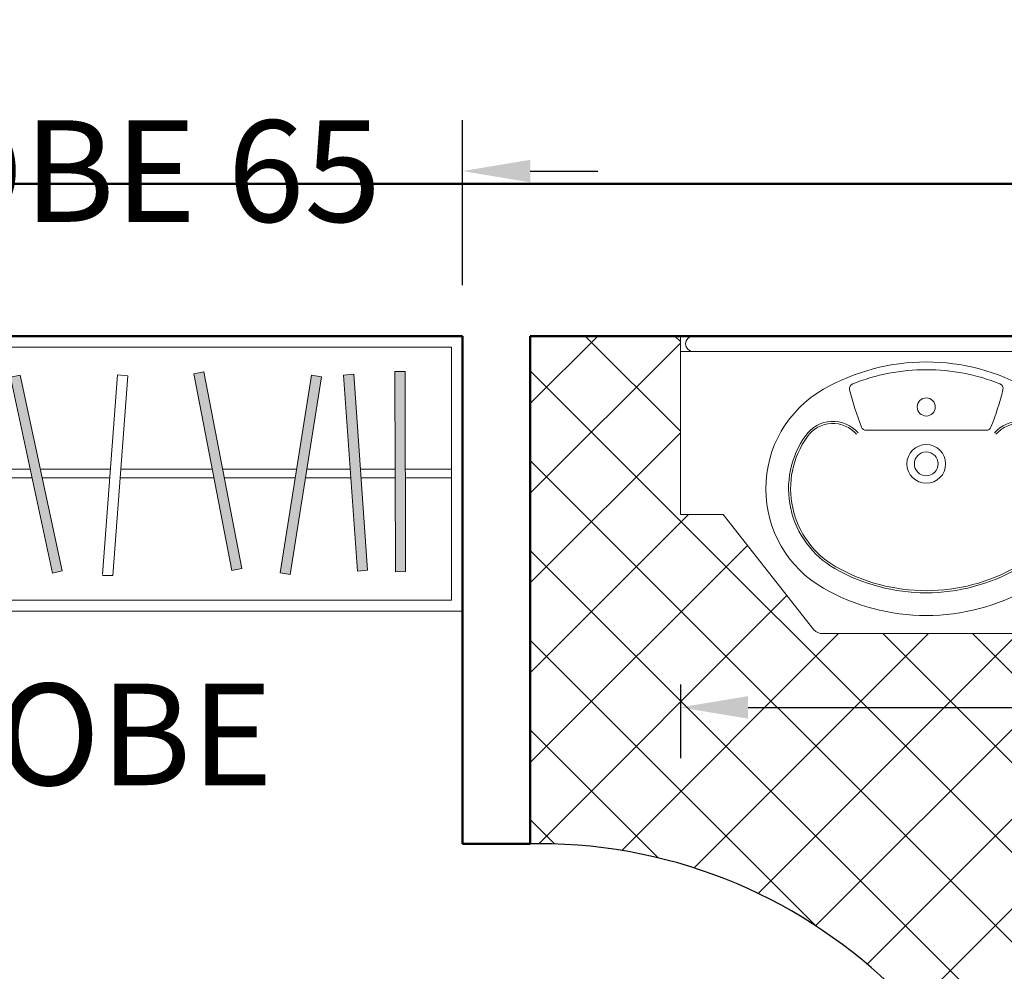
# Model space of a CAD drawing. Units: inches. Extents: x -466983 to 1020, y 324 to 318697.
# Tile 47 of 97: x 491 to 549, y 1038 to 1095. Entities that reach past the tile are written whole.
import ezdxf

# ---------------------------------------------------------------- set-up
doc = ezdxf.new("R2010")
doc.units = ezdxf.units.IN
doc.header["$MEASUREMENT"] = 0
for name, color, linetype, lineweight in [('A-ANNO-DIMS', 2, 'Continuous', 18), ('A-ANNO-TEXT', 7, 'Continuous', 18), ('A-DOOR', 3, 'Continuous', 25), ('A-FLOR-FIXT', 9, 'Continuous', 18), ('A-FLOR-PATT', 252, 'Continuous', 13), ('A-FURN', 8, 'Continuous', 18), ('A-WALL', 7, 'Continuous', 50)]:
    doc.layers.add(name, color=color, linetype=linetype, lineweight=lineweight)
doc.styles.get("Standard").update_dxf_attribs({"font": 'arial.ttf'})
doc.dimstyles.get("Standard").update_dxf_attribs({"dimtxt": 6, "dimasz": 4, "dimexe": 3, "dimexo": 3, "dimgap": 0.09, "dimtad": 0, "dimtih": 1, "dimtoh": 1, "dimdec": 1, "dimzin": 0, "dimdsep": 46, "dimlunit": 3, "dimtxsty": 'Standard', "dimcen": 0.09, "dimadec": 0, "dimazin": 0, "dimtfac": 1, "dimtdec": 1, "dimtofl": 0, "dimtmove": 0, "dimatfit": 3, "dimfxl": 1, "dimtolj": 1, "dimtzin": 0, "dimarcsym": 0})

# ---------------------------------------------------------------- blocks, each defined once
blk = doc.blocks.new('*U38')
for p, q in [((0, 0), (-1.1e-15, 5.999999999999999)), ((40, 8e-15), (40, 6.000000000000007))]:
    blk.add_line(p, q)
blk.add_lwpolyline([(0, 0), (1.42e-14, -40), (1.750000000000014, -40), (1.75, 9e-16)], close=True)
blk.add_arc((0, 0), 40, 270, 0)
blk = doc.blocks.new('B3')
for p, q in [((-450, 0), (-455.7402514854766, -1.1418070123309)), ((450, 0), (455.7402514854766, -1.1418070123309)), ((-463.8581929876745, -9.25974851452338), (-465, -15)), ((-465, -15), (-463.8581929876745, -20.74025148547662)), ((-460.6066017178018, -4.393398282201815), (-463.8581929876745, -9.25974851452338)), ((-455.7402514854766, -1.1418070123309), (-460.6066017178018, -4.393398282201815)), ((455.7402514854766, -1.1418070123309), (460.6066017177945, -4.393398282201815)), ((460.6066017177945, -4.393398282201815), (463.8581929876672, -9.25974851452338)), ((463.8581929876672, -9.25974851452338), (465, -15)), ((465, -15), (463.8581929876672, -20.74025148547662)), ((475, -30), (-475, -30)), ((-463.8581929876745, -20.74025148547662), (-460.6066017178018, -25.60660171779819)), ((-460.6066017178018, -25.60660171779819), (-455.7402514854766, -28.8581929876691)), ((-455.7402514854766, -28.8581929876691), (-450, -30)), ((455.7402514854766, -28.8581929876691), (450, -30)), ((460.6066017177945, -25.60660171779819), (455.7402514854766, -28.8581929876691)), ((463.8581929876672, -20.74025148547662), (460.6066017177945, -25.60660171779819)), ((2.91038e-11, -182.0000000000054), (-115.8117069986983, -182.0000000000054)), ((2.91038e-11, -182.0000000000054), (115.8117069987565, -182.0000000000054))]:
    blk.add_line(p, q)
blk.add_lwpolyline([(199.4833683843535, -575, 0.2017697719241106), (217.3542190239823, -567.482353886593), (392.5, -345), (435, -345), (475, -345), (475, 0), (-475, 0), (-475, -345), (-435, -345), (-392.5, -345), (-217.3542190239896, -567.482353886593, 0.2017697719241107), (-199.4833683843608, -575)], format="xyb", close=True)
for centre, radius, start, end in [((5.09317e-11, -450.0000000000327), 400.0000000000322, 90, 119.7172288959075), ((0, -450.0000000000327), 400.0000000000319, 60.28277110409252, 90), ((2.91038e-11, -450.0000000000055), 385, 90, 111.6513567404431), ((2.91038e-11, -450.0000000000055), 385, 68.34864325955687, 90), ((-138.3591766736499, -101.4576952073475), 10, 111.6513567404431, 193.3915177581575), ((138.3591766737008, -101.4576952073475), 10, 346.6084822418425, 68.34864325955687), ((-88.47222222221171, -295.0000000000055), 221.527777777762, 119.7172288959075, 240.2827711040925), ((338.3178096717893, 12.0282100348104), 500, 193.3915177581575, 202.0594091764406), ((-338.3178096717383, 12.0282100348104), 500, 337.9405908235594, 346.6084822418425), ((88.47222222225537, -294.9999999999964), 221.527777777762, 299.7172288959074, 60.28277110409252), ((2.91038e-11, -136.9999999999891), 17.5, 90, 270), ((2.91038e-11, -136.9999999999891), 17.5, 270, 90), ((-180.5137974189128, -229.2550553338115), 64.41699441097052, 40.71477974361456, 144.4619255202982), ((-180.5137974189128, -229.2550553338115), 60.41699441097051, 40.71477974361456, 144.4619255202982), ((180.5137974189638, -229.2550553338115), 64.41699441097052, 35.53807447970174, 139.2852202563854), ((180.5137974189638, -229.2550553338115), 60.41699441097051, 35.53807447970174, 139.2852202563854), ((-115.8117069986983, -172.0000000000145), 10, 202.0594091764406, 270), ((115.8117069987565, -172.0000000000145), 10, 270, 337.9405908235594), ((-88.47222222221171, -295.0000000000055), 177.5277777777778, 144.4619255202982, 240.2827711040925), ((-88.47222222221171, -295.0000000000055), 173.5277777777778, 144.4619255202982, 240.2827711040925), ((88.47222222223354, -295.0000000000055), 173.5277777777778, 299.7172288959074, 35.53807447970174), ((88.47222222223354, -295.0000000000055), 177.5277777777778, 299.7172288959074, 35.53807447970174), ((2.91038e-11, -247.0000000000037), 37.5, 90, 270), ((2.91038e-11, -247.0000000000037), 23, 90, 270), ((2.91038e-11, -247.0000000000037), 37.5, 270, 90), ((2.91038e-11, -247.0000000000037), 23, 270, 90), ((2.91038e-11, -140.0000000000036), 356, 240.2827711040925, 270), ((2.91038e-11, -140.0000000000036), 352, 240.2827711040925, 270), ((2.91038e-11, -140.0000000000036), 352, 270, 299.7172288959074), ((2.91038e-11, -140.0000000000036), 356, 270, 299.7172288959074), ((5.09317e-11, -139.9999999999781), 400.0000000000309, 240.2827711040925, 270), ((-1.45519e-11, -140.0000000000309), 399.9999999999781, 270, 299.7172288959074)]:
    blk.add_arc(centre, radius, start, end)
blk = doc.blocks.new('Wardrobe 1.1')
h = blk.add_hatch(color=256)
h.dxf.hatch_style = 1
h.paths.add_polyline_path([(4623.63130591675, 1559.127828082639), (4605.452274823494, 1555.618178042687), (4674.43862754123, 1198.026895294012), (4692.617658634486, 1201.536545333964)])
h = blk.add_hatch(color=256)
h.dxf.hatch_style = 1
h.paths.add_polyline_path([(4989.37316691601, 1559.911022331437), (4970.858516418657, 1559.860704815934), (4971.798831744867, 1195.677017418713), (4990.313482242336, 1195.727334934216)])
h = blk.add_hatch(color=256)
h.dxf.hatch_style = 1
h.paths.add_polyline_path([(3151.282105115228, 1187.510288244974), (3169.796885531561, 1187.510288244974), (3168.856570205235, 1551.693975642194), (3150.341919707882, 1551.643658126692)])
h = blk.add_hatch(color=256)
h.dxf.hatch_style = 1
h.paths.add_polyline_path([(3361.868584936534, 1541.669378461711), (3343.939726713163, 1546.290077294676), (3253.002619132332, 1193.641406768397), (3270.931477355587, 1189.02070793549)])
h = blk.add_hatch(color=256)
h.dxf.hatch_style = 1
h.paths.add_polyline_path([(3403.891248248334, 1551.693975642194), (3385.376597750981, 1551.643658126692), (3386.316913077191, 1187.459970729471), (3404.831563574544, 1187.510288244974)])
h = blk.add_hatch(color=256)
h.dxf.hatch_style = 1
h.paths.add_polyline_path([(3596.9032629794, 1541.669378461711), (3578.974404756262, 1546.290077294676), (3488.037297175316, 1193.641406768397), (3505.966155398454, 1189.02070793549)])
h = blk.add_hatch(color=256)
h.dxf.hatch_style = 1
h.paths.add_polyline_path([(3664.213577620618, 1553.074679382599), (3646.111361609239, 1549.18821693327), (3722.509827192224, 1193.106882382172), (3740.612043203603, 1196.993344831501)])
h = blk.add_hatch(color=256)
h.dxf.hatch_style = 1
h.paths.add_polyline_path([(3813.833679657712, 1190.320201264565), (3832.296488257873, 1188.934736184298), (3859.597907476409, 1552.094859088468), (3841.135098876248, 1553.480324168735)])
h = blk.add_hatch(color=256)
h.dxf.hatch_style = 1
h.paths.add_polyline_path([(4029.392729275909, 1551.693975642194), (4010.878078778556, 1551.643658126692), (4011.818394104767, 1187.459970729471), (4030.333044602236, 1187.510288244974)])
h = blk.add_hatch(color=256)
h.dxf.hatch_style = 1
h.paths.add_polyline_path([(4222.404744007092, 1541.669378461711), (4204.475885783836, 1546.290077294676), (4113.538778203007, 1193.641406768397), (4131.467636426145, 1189.02070793549)])
h = blk.add_hatch(color=256)
h.dxf.hatch_style = 1
h.paths.add_polyline_path([(4348.011308219915, 1193.106882382172), (4366.113524231294, 1196.993344831501), (4289.715058648309, 1553.074679382599), (4271.612842636931, 1549.18821693327)])
h = blk.add_hatch(color=256)
h.dxf.hatch_style = 1
h.paths.add_polyline_path([(4837.600952654661, 1550.260731044678), (4819.316543353771, 1553.17194924514), (4762.004005428219, 1193.525017719703), (4780.288414729109, 1190.613799519242)])
h = blk.add_hatch(color=256)
h.dxf.hatch_style = 1
h.paths.add_polyline_path([(4895.873954488479, 1554.659198605851), (4877.410424046501, 1553.283386659738), (4902.671188982951, 1196.772307061869), (4921.13471942493, 1198.148119007923)])
at = {"ltscale": 5}
for p, q in [((3093.82979383441, 1124.111993690416), (3093.82979383441, 1624.111993690416)), ((3093.82979383441, 1624.111993690416), (5093.829793834409, 1624.111993690416)), ((5093.829793834409, 1624.111993690416), (5093.829793834409, 1124.111993690416)), ((5093.829793834409, 1124.111993690416), (3093.82979383441, 1124.111993690416))]:
    blk.add_line(p, q, dxfattribs=at)
for p, q in [((3113.82979383441, 1144.111993690416), (3113.82979383441, 1604.111993690416)), ((3113.82979383441, 1604.111993690416), (5073.829793834409, 1604.111993690416)), ((5073.829793834409, 1604.111993690416), (5073.829793834409, 1144.111993690416)), ((4623.63130591675, 1559.127828082639), (4605.452274823494, 1555.618178042687)), ((4692.617658634486, 1201.536545333964), (4623.63130591675, 1559.127828082639)), ((4989.37316691601, 1559.911022331437), (4970.858516418657, 1559.860704815934)), ((4970.858516418657, 1559.860704815934), (4971.798831744867, 1195.677017418713)), ((4990.313482242336, 1195.727334934216), (4989.37316691601, 1559.911022331437)), ((3168.856570205235, 1551.693975642194), (3150.341919707882, 1551.643658126692)), ((3150.341919707882, 1551.643658126692), (3151.282235034092, 1187.459970729471)), ((3169.796885531561, 1187.510288244974), (3168.856570205235, 1551.693975642194)), ((3343.939726713163, 1546.290077294676), (3253.002619132332, 1193.641406768397)), ((3270.931477355587, 1189.02070793549), (3361.868584936534, 1541.669378461711)), ((3361.868584936534, 1541.669378461711), (3343.939726713163, 1546.290077294676)), ((3403.891248248334, 1551.693975642194), (3385.376597750981, 1551.643658126692)), ((3385.376597750981, 1551.643658126692), (3386.316913077191, 1187.459970729471)), ((3404.831563574544, 1187.510288244974), (3403.891248248334, 1551.693975642194)), ((3578.974404756262, 1546.290077294676), (3488.037297175316, 1193.641406768397)), ((3505.966155398454, 1189.02070793549), (3596.9032629794, 1541.669378461711)), ((3596.9032629794, 1541.669378461711), (3578.974404756262, 1546.290077294676)), ((3664.213577620618, 1553.074679382599), (3646.111361609239, 1549.18821693327)), ((3646.111361609239, 1549.18821693327), (3722.509827192224, 1193.106882382172)), ((3740.612043203603, 1196.993344831501), (3664.213577620618, 1553.074679382599)), ((3841.135098876248, 1553.480324168735), (3813.833679657712, 1190.320201264565)), ((3832.296488257873, 1188.934736184298), (3859.597907476409, 1552.094859088468)), ((3859.597907476409, 1552.094859088468), (3841.135098876248, 1553.480324168735)), ((4029.392729275909, 1551.693975642194), (4010.878078778556, 1551.643658126692)), ((4010.878078778556, 1551.643658126692), (4011.818394104767, 1187.459970729471)), ((4030.333044602236, 1187.510288244974), (4029.392729275909, 1551.693975642194)), ((4204.475885783836, 1546.290077294676), (4113.538778203007, 1193.641406768397)), ((4131.467636426145, 1189.02070793549), (4222.404744007092, 1541.669378461711)), ((4222.404744007092, 1541.669378461711), (4204.475885783836, 1546.290077294676)), ((4289.715058648309, 1553.074679382599), (4271.612842636931, 1549.18821693327)), ((4271.612842636931, 1549.18821693327), (4348.011308219915, 1193.106882382172)), ((4366.113524231294, 1196.993344831501), (4289.715058648309, 1553.074679382599)), ((4605.452274823494, 1555.618178042687), (4674.43862754123, 1198.026895294012)), ((4819.316543353771, 1553.17194924514), (4762.004005428219, 1193.525017719703)), ((4780.288414729109, 1190.613799519242), (4837.600952654661, 1550.260731044678)), ((4837.600952654661, 1550.260731044678), (4819.316543353771, 1553.17194924514)), ((4895.873954488479, 1554.659198605851), (4877.410424046501, 1553.283386659738)), ((4877.410424046501, 1553.283386659738), (4902.671188982951, 1196.772307061869)), ((4921.13471942493, 1198.148119007923), (4895.873954488479, 1554.659198605851)), ((3150.779647227988, 1382.111993690416), (3113.82979383441, 1382.111993690416)), ((3301.603312885615, 1382.111993690416), (3169.294427644258, 1382.111993690416)), ((3301.603312885671, 1382.111993690416), (3169.294427644278, 1382.111993690416)), ((3385.814325271087, 1382.111993690416), (3320.723705409183, 1382.111993690416)), ((3536.63799092866, 1382.111993690416), (3404.329105687303, 1382.111993690416)), ((3536.637990928537, 1382.111993690416), (3404.329105687377, 1382.111993690416)), ((3681.958135513426, 1382.111993690416), (3555.75838345205, 1382.111993690416)), ((3681.958135513406, 1382.111993690416), (3555.758383452127, 1382.111993690416)), ((3828.252080240405, 1382.111993690416), (3700.894205307252, 1382.111993690416)), ((3828.252080240453, 1382.111993690416), (3700.894205307288, 1382.111993690416)), ((4011.315806298681, 1382.111993690416), (3846.819044447374, 1382.111993690416)), ((4162.139471956229, 1382.111993690416), (4029.830586714952, 1382.111993690416)), ((4307.459616541096, 1382.111993690416), (4181.259864479818, 1382.111993690416)), ((4453.753561268143, 1382.111993690416), (4326.395686334979, 1382.111993690416)), ((4638.925011464094, 1382.111993690416), (4472.320525475011, 1382.111993690416)), ((4792.056807955193, 1382.111993690416), (4657.781122696752, 1382.111993690416)), ((4889.538855865531, 1382.111993690416), (4810.805142536459, 1382.111993690416)), ((4971.317460196375, 1382.111993690416), (4908.099870128257, 1382.111993690416)), ((5073.829793834409, 1382.111993690416), (4989.832240612645, 1382.111993690416)), ((3150.820958922443, 1366.111993690417), (3113.82979383441, 1366.111993690416)), ((3297.477411264826, 1366.111993690417), (3169.335739338719, 1366.111993690417)), ((3297.477411264836, 1366.111993690416), (3169.33573933882, 1366.111993690416)), ((3385.855636965543, 1366.111993690416), (3316.597803788389, 1366.111993690416)), ((3532.512089307866, 1366.111993690416), (3404.370417381759, 1366.111993690416)), ((3532.512089307935, 1366.111993690416), (3404.370417381687, 1366.111993690416)), ((3685.390990119154, 1366.111993690416), (3551.632481831255, 1366.111993690417)), ((3685.390990119244, 1366.111993690416), (3551.632481831408, 1366.111993690416)), ((3827.049242483872, 1366.111993690416), (3704.32705991298, 1366.111993690416)), ((3827.049242483967, 1366.111993690416), (3704.327059913011, 1366.111993690416)), ((4011.357117993108, 1366.111993690416), (3845.61620669084, 1366.111993690416)), ((4158.013570335509, 1366.111993690416), (4029.871898409377, 1366.111993690416)), ((4310.892471146819, 1366.111993690416), (4177.133962858983, 1366.111993690416)), ((4452.550723511541, 1366.111993690416), (4329.828540940702, 1366.111993690416)), ((4642.011724414702, 1366.111993690416), (4471.117687718526, 1366.111993690416)), ((4789.507083415918, 1366.111993690416), (4660.867835647359, 1366.111993690416)), ((4890.672543602346, 1366.111993690416), (4808.255417997067, 1366.111993690416)), ((4971.3587718908, 1366.111993690416), (4909.233557865072, 1366.111993690416)), ((5073.829793834409, 1366.111993690416), (4989.873552307186, 1366.111993690416)), ((4674.43862754123, 1198.026895294012), (4692.617658634486, 1201.536545333964)), ((3169.796885531561, 1187.510288244974), (3151.282105115229, 1187.510288244974)), ((3253.002619132332, 1193.641406768397), (3270.931477355587, 1189.02070793549)), ((3404.831563574544, 1187.510288244974), (3386.316913077191, 1187.459970729471)), ((3488.037297175316, 1193.641406768397), (3505.966155398454, 1189.02070793549)), ((3722.509827192224, 1193.106882382172), (3740.612043203603, 1196.993344831501)), ((3832.296488257873, 1188.934736184298), (3813.833679657712, 1190.320201264565)), ((4030.333044602236, 1187.510288244974), (4011.818394104767, 1187.459970729471)), ((4113.538778203007, 1193.641406768397), (4131.467636426145, 1189.02070793549)), ((4348.011308219915, 1193.106882382172), (4366.113524231294, 1196.993344831501)), ((4762.004005428219, 1193.525017719703), (4780.288414729109, 1190.613799519242)), ((4902.671188982951, 1196.772307061869), (4921.13471942493, 1198.148119007923)), ((4971.798831744867, 1195.677017418713), (4990.313482242336, 1195.727334934216)), ((5073.829793834409, 1144.111993690416), (3113.82979383441, 1144.111993690416))]:
    blk.add_line(p, q)
blk.add_lwpolyline([(4439.335160685403, 1190.320201264565), (4466.63657990394, 1553.480324168735), (4485.0993885041, 1552.094859088468), (4457.797969285564, 1188.934736184298), (4439.231005078596, 1188.934736184298)])
blk = doc.blocks.new('*D79')
at = {"layer": 'A-ANNO-DIMS', "color": 0, "lineweight": -2, "transparency": 16777216}
for p, q in [((529.6742726119846, 1055.350891982691), (529.6742726119846, 1050.992414036445)), ((558.7307922536265, 1055.350891982691), (558.7307922536265, 1050.992414036445)), ((533.6742726119846, 1053.992414036445), (554.7307922536265, 1053.992414036445)), ((558.7307922536265, 1053.992414036445), (562.7307922536265, 1053.992414036445))]:
    blk.add_line(p, q, dxfattribs=at)
at = {"layer": 'A-ANNO-DIMS', "color": 0, "transparency": 16777216}
for points in [[(533.6742726119846, 1054.659080703112), (533.6742726119846, 1053.325747369778), (529.6742726119846, 1053.992414036445)], [(554.7307922536265, 1054.659080703112), (554.7307922536265, 1053.325747369778), (558.7307922536265, 1053.992414036445)]]:
    blk.add_solid(points, dxfattribs=at)
at = {"layer": 'Defpoints', "color": 0, "transparency": 16777216}
for p in [(529.6742726119846, 1058.350891982691), (558.7307922536265, 1058.350891982691), (558.7307922536265, 1053.992414036445)]:
    blk.add_point(p, dxfattribs=at)
at = {"layer": 'A-ANNO-DIMS', "color": 0, "transparency": 16777216, "insert": (603.861037819793, 1053.992414036445), "char_height": 6, "attachment_point": 5}
blk.add_mtext('\\A1;WASHBASIN 29 TYP.', dxfattribs=at)
blk = doc.blocks.new('*D83')
at = {"layer": 'A-ANNO-DIMS', "color": 0, "lineweight": -2, "transparency": 16777216}
for p, q in [((451.8056775209043, 1078.937732818421), (451.8056775209043, 1088.687732818421)), ((516.8056775209042, 1078.937732818421), (516.8056775209042, 1088.687732818421)), ((447.8056775209043, 1085.687732818422), (443.8056775209043, 1085.687732818422)), ((520.8056775209042, 1085.687732818422), (524.8056775209042, 1085.687732818422))]:
    blk.add_line(p, q, dxfattribs=at)
at = {"layer": 'A-ANNO-DIMS', "color": 0, "transparency": 16777216}
for points in [[(447.8056775209043, 1086.354399485088), (447.8056775209043, 1085.021066151755), (451.8056775209043, 1085.687732818422)], [(520.8056775209042, 1086.354399485088), (520.8056775209042, 1085.021066151755), (516.8056775209042, 1085.687732818422)]]:
    blk.add_solid(points, dxfattribs=at)
at = {"layer": 'Defpoints', "color": 0, "transparency": 16777216}
for p in [(516.8056775209042, 1085.687732818422), (451.8056775209043, 1075.937732818421), (516.8056775209042, 1075.937732818421)]:
    blk.add_point(p, dxfattribs=at)
at = {"layer": 'A-ANNO-DIMS', "color": 0, "transparency": 16777216, "insert": (484.3056775209042, 1085.687732818422), "char_height": 6, "attachment_point": 5}
blk.add_mtext('\\A1;WARDROBE 65', dxfattribs=at)

msp = doc.modelspace()

# ---------------------------------------------------------------- hatches: boundary and pattern name
at = {"layer": 'A-FLOR-PATT', "transparency": 33554572}
h = msp.add_hatch(dxfattribs=at)
h.set_pattern_fill('ANSI37', color=256, scale=30)
h.set_pattern_definition([(45, (-1212.413693079869, -290.0350025265127), (-2.651650429449553, 2.651650429449553), []), (135, (-1212.413693079869, -290.0350025265127), (-2.651650429449553, -2.651650429449552), [])])
h.paths.add_polyline_path([(901.805677520904, 1075.937732818422), (900.6144036774049, 1075.937732818422), (900.6144036774049, 1065.385628316983), (899.390971271441, 1065.385628316983), (898.0910743401043, 1065.385628316983), (892.8355944880973, 1058.709752245277, -0.2583770168556315), (892.18750428989, 1058.350891982691), (879.9847834232776, 1058.350891982691, -0.2017697719240963), (879.438188978411, 1058.580825279484), (874.0812133730635, 1065.385628316983), (872.7813164417267, 1065.385628316983), (871.5578840357629, 1065.385628316983), (871.5578840357629, 1075.937732818422), (813.8056775209042, 1075.937732818422), (813.8056775209042, 1044.792233318721), (832.3947444543938, 1044.792233318721, -0.3947951267487684), (848.6601780212009, 1028.535584015862), (848.6601780212009, 1009.937732818421), (901.805677520904, 1009.937732818421), (901.805677520904, 1015.937732818421), (901.3056775209042, 1015.937732818421), (871.3056775209039, 1015.937732818421), (871.3056775209039, 1017.250232818421), (871.3344022102003, 1017.250232818421, -0.4014527144963572), (901.3056775209042, 1045.937732818421), (901.805677520904, 1045.937732818421)])
edge = h.paths.add_edge_path(flags=16)
edge.add_line((847.7730719745084, 1068.948588737025), (847.7730719745069, 1073.708823774771))
edge.add_arc((849.2268986539951, 1073.708823774771), 1.453826679487974, 90, 180, ccw=False)
edge.add_line((849.2268986539951, 1075.162650454259), (864.4920787886183, 1075.162650454259))
edge.add_arc((864.4920787886213, 1073.708823774771), 1.453826679487974, 0, 90.00000000012102, ccw=False)
edge.add_line((865.9459054681093, 1073.708823774771), (865.9459054681081, 1069.00351244647))
edge.add_arc((832.6447385074767, 1068.976050591752), 33.30117828385809, -20.61233806670998, 0.04724903539101888, ccw=False)
edge.add_ellipse((856.8594887213083, 1058.479989307073), major_axis=(-2.091e-13, 10.21313242340307), ratio=0.6859192225533502, start_angle=100.00884331843292, end_angle=259.9911566815624, ccw=False)
edge.add_arc((881.0742389351396, 1068.976050591752), 33.30117828385809, 180.0472490354062, 200.6123380667097, ccw=False)
h.paths.add_polyline_path([(853.145578187156, 1066.481532374271), (853.145578187156, 1066.453444752512), (853.1463399851561, 1066.453444752512, 0.4331071439582673), (852.9166149812349, 1066.684892837266), (852.9166149812349, 1066.453444752512), (853.145578187156, 1066.453444752512), (853.145578187156, 1066.481532374489), (853.088019486549, 1066.612171966583, 0.6979386910037918), (852.699540939094, 1066.453444752512), (852.7003027371272, 1066.453444752512), (852.7003027371272, 1066.481532374489), (852.9166149812349, 1067.001204630995), (852.9166149812349, 1066.684892837266, -0.3962543063594317)], flags=0)
h.paths.add_polyline_path([(861.0186747055222, 1066.481532374271), (861.0186747055222, 1066.453444752512), (861.0194365035225, 1066.453444752512, 0.4164039232557909), (860.8023624614146, 1066.684892837265), (860.8023624614146, 1066.453444752512), (861.0186747055222, 1066.453444752512), (861.0186747055222, 1066.481532374489), (860.9671752720659, 1066.605255499379, 0.7133437187663149), (860.5726374574602, 1066.453444752512), (860.5733992554934, 1066.453444752512), (860.5733992554934, 1066.481532374489), (860.8023624614146, 1067.001204630995), (860.8023624614146, 1066.684892837265, -0.3799725304814568)], flags=0)
edge = h.paths.add_edge_path(flags=0)
edge.add_spline(control_points=[(861.1298377106021, 1065.785468371534), (861.4660965533383, 1065.247811229462), (861.613385559155, 1065.016139861057), (861.9832837951076, 1064.373617117607), (862.1924105327118, 1063.944313665492), (862.5613774174725, 1063.039129539609), (862.7212131906668, 1062.56326642291), (862.9865156700853, 1061.578122280975), (863.0919804897928, 1061.068856600952), (863.2452407883674, 1060.031049745086), (863.293035446714, 1059.502522766744), (863.3294736797056, 1058.440879580113), (863.3181170778639, 1057.907777155726), (863.2366033468288, 1056.85179603536), (863.1664466211855, 1056.328931215311), (862.9695120306455, 1055.307951977375), (862.8427353108815, 1054.809852090196), (862.5365466723708, 1053.852219447362), (862.3571373353129, 1053.392702749349), (861.9514237071658, 1052.524888245794), (861.7251255454219, 1052.116609101398), (861.2330086320977, 1051.362239687588), (860.9672044472572, 1051.016170456457), (860.4047960485765, 1050.394909316517), (860.1082220871676, 1050.119734477926), (859.493696255806, 1049.64606200509), (859.1757900615103, 1049.447558762665), (858.5275631429041, 1049.129883644436), (858.197273503909, 1049.010664382187), (857.5314773710529, 1048.851811036626), (857.1959384637446, 1048.812116564677), (856.5249326641573, 1048.811967422545), (856.1893892160524, 1048.851512676201), (855.5235728169741, 1049.010066967686), (855.1932673158994, 1049.129136347874), (854.5449932971788, 1049.446513839261), (854.2270557868354, 1049.644869411481), (853.6124495619564, 1050.118254324803), (853.3158265363004, 1050.393289340464), (852.7533025914207, 1051.014284587242), (852.487431959371, 1051.360227769297), (851.9951668313728, 1052.114363776776), (851.7687869247744, 1052.522535562859), (851.3628973914427, 1053.390157753425), (851.1833939042357, 1053.849589492002), (850.8770077813263, 1054.807077270704), (850.7501277313783, 1055.30511724975), (850.5529806633081, 1056.326003473117), (850.4827147921034, 1056.848835185142), (850.4009803807432, 1057.904777820697), (850.3895122452288, 1058.437874867502), (850.425728471152, 1059.499535178563), (850.4734126571939, 1060.02808465918), (850.6264565107679, 1061.065963770327), (850.7318153592672, 1061.575279204679), (850.9969137893603, 1062.560548677974), (851.1566514873134, 1063.036487374614), (851.525433403113, 1063.94184619004), (851.7344732542367, 1064.371248757046), (852.1056260411488, 1065.016350037675), (852.2544071072941, 1065.250281998093), (852.608154630964, 1065.733465727338)], knot_values=[3.915332106759953, 3.915332106759953, 3.915332106759953, 3.915332106759953, 4.013467662305501, 4.013467662305501, 4.175531746215815, 4.175531746215815, 4.337595830126129, 4.337595830126129, 4.499659914036444, 4.499659914036444, 4.661723997946757, 4.661723997946757, 4.82378808185707, 4.82378808185707, 4.985852165767384, 4.985852165767384, 5.147916249677697, 5.147916249677697, 5.30998033358801, 5.30998033358801, 5.472044417498324, 5.472044417498324, 5.634108501408637, 5.634108501408637, 5.79617258531895, 5.79617258531895, 5.958236669229264, 5.958236669229264, 6.120300753139577, 6.120300753139577, 6.282364837049891, 6.282364837049891, 6.444428920960204, 6.444428920960204, 6.606493004870517, 6.606493004870517, 6.768557088780831, 6.768557088780831, 6.930621172691144, 6.930621172691144, 7.092685256601457, 7.092685256601457, 7.254749340511771, 7.254749340511771, 7.416813424422084, 7.416813424422084, 7.578877508332397, 7.578877508332397, 7.740941592242711, 7.740941592242711, 7.903005676153024, 7.903005676153024, 8.065069760063338, 8.065069760063338, 8.22713384397365, 8.22713384397365, 8.389197927883965, 8.389197927883965, 8.551262011794279, 8.551262011794279, 8.650370494357087, 8.650370494357087, 8.650370494357087, 8.650370494357087], degree=3, periodic=0)
edge.add_line((852.6421178657537, 1065.785468371534), (861.1298377106024, 1065.785468371534))
edge = h.paths.add_edge_path(flags=0)
edge.add_ellipse((856.8495804607978, 1057.743205248224), major_axis=(-3.1e-13, 7.792134415209829), ratio=0.6878610933899516, start_angle=0, end_angle=360)
h.paths.add_polyline_path([(848.8634419841151, 1069.389059844444), (848.863441984139, 1073.960453158315, -0.4142135623709757), (849.9538119937549, 1075.050823167924), (863.765165448898, 1075.050823167924, -0.4142135623721942), (864.8555354585106, 1073.960453158308), (864.8555354584933, 1069.389059844444, -0.3889362887010341), (864.5236837164459, 1069.026979909221, -0.0435607626104464), (849.19529372618, 1069.02697990933, -0.3889362886276668)], flags=0)
h.paths.add_polyline_path([(853.1006153779753, 1068.112209480768, -1), (852.677499999749, 1068.112209480768, -1)], flags=0)
edge = h.paths.add_edge_path(flags=0)
edge.add_ellipse((856.8594887213083, 1057.33782914961), major_axis=(7.74e-14, 2.20702192546696), ratio=0.6571642650458812, start_angle=0, end_angle=360)
h.paths.add_polyline_path([(861.0414774428674, 1068.112209480768, -1), (860.6183620646412, 1068.112209480768, -1)], flags=0)
edge = h.paths.add_edge_path()
edge.add_line((573.9536545579417, 1057.341203598636), (573.9536545579417, 1075.937732818422))
edge.add_line((573.9536545579417, 1075.937732818422), (558.7307922536265, 1075.937732818422))
edge.add_line((558.7307922536265, 1075.937732818422), (558.7307922536265, 1065.385628316983))
edge.add_line((558.7307922536265, 1065.385628316983), (557.5073598476627, 1065.385628316983))
edge.add_line((557.5073598476627, 1065.385628316983), (556.207462916326, 1065.385628316983))
edge.add_line((556.207462916326, 1065.385628316983), (550.9519830643189, 1058.709752245277))
edge.add_arc((550.3038928661116, 1059.115537236419), 0.7646452537275144, 270, 327.94831933647396, ccw=False)
edge.add_line((550.3038928661116, 1058.350891982691), (538.1011719994992, 1058.350891982691))
edge.add_arc((538.1011719994992, 1059.115537236419), 0.7646452537275137, 224.3704013916024, 270, ccw=False)
edge.add_line((537.5545775546327, 1058.580825279484), (532.1976019492852, 1065.385628316983))
edge.add_line((532.1976019492852, 1065.385628316983), (530.8977050179485, 1065.385628316983))
edge.add_line((530.8977050179485, 1065.385628316983), (529.6742726119846, 1065.385628316983))
edge.add_line((529.6742726119846, 1065.385628316983), (529.6742726119846, 1075.937732818422))
edge.add_line((529.6742726119846, 1075.937732818422), (520.8056775209042, 1075.937732818422))
edge.add_line((520.8056775209042, 1075.937732818422), (520.8056775209042, 1045.937732818422))
edge.add_line((520.8056775209042, 1045.937732818422), (521.3056775209044, 1045.937732818422))
edge.add_arc((521.3056775209042, 1015.937732818422), 30.00000000000023, 2.507490703587223, 89.99999999999977, ccw=False)
edge.add_line((551.2769528316082, 1017.250232818422), (551.3056775209045, 1017.250232818422))
edge.add_line((551.3056775209045, 1017.250232818422), (551.3056775209045, 1015.937732818422))
edge.add_line((551.3056775209045, 1015.937732818422), (520.8056775209042, 1015.937732818422))
edge.add_line((520.8056775209042, 1015.937732818422), (520.8056775209042, 1009.937732818421))
edge.add_line((520.8056775209042, 1009.937732818421), (559.1912990237018, 1010.402158339383))
edge.add_arc((559.1912990237018, 1011.855985018871), 1.453826679487974, 180, 270, ccw=False)
edge.add_line((557.7374723442138, 1011.855985018871), (557.7374723442151, 1016.561296347171))
edge.add_arc((591.0386393048469, 1016.58875820189), 33.3011782838587, 159.3876619332891, 180.0472490353913, ccw=False)
edge.add_ellipse((566.8238890910148, 1027.084819486569), major_axis=(-3.171e-13, 10.21313242340307), ratio=0.6859192225533445, start_angle=280.00884331843395, end_angle=439.99115668156304, ccw=False)
edge.add_arc((542.6091388771833, 1016.58875820189), 33.3011782838584, 0.04724903544490644, 20.612338066710322, ccw=False)
edge.add_line((575.9103058378148, 1016.61622005664), (575.910305837816, 1011.855985018871))
edge.add_arc((574.4564791583282, 1011.855985018871), 1.453826679487974, -90, 0, ccw=False)
edge.add_line((574.4564791583282, 1010.402158339383), (608.8056775209044, 1009.937732818421))
edge.add_line((608.8056775209044, 1009.937732818421), (608.8056775209044, 1041.08570985546))
edge.add_line((608.8056775209044, 1041.08570985546), (590.2179319406538, 1041.08570985546))
edge.add_arc((590.7750219589672, 1057.907380652626), 16.83089295601249, 181.9277454211679, 268.1032059320871, ccw=False)
edge = h.paths.add_edge_path()
edge.add_ellipse((494.2443328575609, 583.6203939656394), major_axis=(-2.099e-13, 10.21313242340307), ratio=0.6859192225533391, start_angle=280.0088433184392, end_angle=439.99115668155895, ccw=False)
edge.add_arc((470.0295826437295, 573.1243326809605), 33.30117828385828, 0.047249035653180727, 20.612338066711573, ccw=False)
edge.add_line((503.3307496043607, 573.1517945358311), (503.3307496043621, 568.3915594979414))
edge.add_arc((501.8769229248741, 568.3915594979414), 1.453826679487974, -90, 0, ccw=False)
edge.add_line((501.8769229248741, 566.9377328184536), (539.8056775209043, 566.9377328184218))
edge.add_line((539.8056775209043, 566.9377328184218), (539.8056775209043, 572.9377328184218))
edge.add_line((539.8056775209043, 572.9377328184218), (539.3056775209043, 572.9377328184218))
edge.add_line((539.3056775209043, 572.9377328184218), (509.3056775209042, 572.9377328184218))
edge.add_line((509.3056775209042, 572.9377328184218), (509.3056775209042, 574.2502328184218))
edge.add_line((509.3056775209042, 574.2502328184218), (509.3344022102004, 574.2502328184218))
edge.add_arc((539.3056775209043, 572.9377328184218), 30.00000000000003, 90, 177.4925092964128, ccw=False)
edge.add_line((539.3056775209043, 602.9377328184218), (539.8056775209043, 602.9377328184218))
edge.add_line((539.8056775209043, 602.9377328184218), (539.8056775209043, 626.9377328184219))
edge.add_line((539.8056775209043, 626.9377328184219), (531.7718318056131, 626.9377328184219))
edge.add_line((531.7718318056131, 626.9377328184219), (531.7718318056131, 616.3856283169836))
edge.add_line((531.7718318056131, 616.3856283169836), (530.5483993996492, 616.3856283169836))
edge.add_line((530.5483993996492, 616.3856283169836), (529.2485024683125, 616.3856283169836))
edge.add_line((529.2485024683125, 616.3856283169836), (523.7105154427977, 609.3508919826913))
edge.add_line((523.7105154427977, 609.3508919826913), (510.7766285267865, 609.3508919826913))
edge.add_line((510.7766285267865, 609.3508919826913), (505.2386415012717, 616.3856283169835))
edge.add_line((505.2386415012717, 616.3856283169835), (503.9387445699351, 616.3856283169836))
edge.add_line((503.9387445699351, 616.3856283169836), (502.7153121639711, 616.3856283169836))
edge.add_line((502.7153121639711, 616.3856283169836), (502.7153121639712, 626.9377328184219))
edge.add_line((502.7153121639712, 626.9377328184219), (481.698294634846, 626.937732818422))
edge.add_line((481.698294634846, 626.937732818422), (481.6982946348461, 610.9950036909872))
edge.add_arc((467.2703297247223, 611.4728203914133), 14.43587476556121, 271.9277454211847, 358.103205932099, ccw=False)
edge.add_line((467.7559403853078, 597.0451157044822), (451.8056775209041, 597.0451157044822))
edge.add_line((451.8056775209041, 597.0451157044822), (451.8056775209041, 584.4035114605515))
edge.add_line((451.8056775209041, 584.4035114605515), (451.8056775209043, 566.9377328184218))
edge.add_line((451.8056775209043, 566.9377328184218), (486.6117427902477, 566.9377328184536))
edge.add_arc((486.6117427902477, 568.3915594979414), 1.453826679487974, 180, 270, ccw=False)
edge.add_line((485.1579161107598, 568.3915594979414), (485.157916110761, 573.0968708261933))
edge.add_arc((518.4590830713927, 573.1243326809608), 33.3011782838585, 159.387661933289, 180.0472490354759, ccw=False)
h.paths.add_polyline_path([(836.2608886421394, 1020.732838196592), (879.8898108795202, 1020.732838196592), (879.8898108795202, 1039.390182443977), (836.2608886421394, 1039.390182443977)], flags=25)
h.paths.add_polyline_path([(549.9851009445293, 1036.749159167106), (593.6140231819099, 1036.749159167106), (593.6140231819099, 1055.406503414491), (549.9851009445293, 1055.406503414491)], flags=24)
h.paths.add_polyline_path([(475.1230325221868, 595.5958681380167), (518.7519547595675, 595.5958681380167), (518.7519547595675, 614.2532123854019), (475.1230325221868, 614.2532123854019)], flags=24)

# ---------------------------------------------------------------- linework, layer by layer
at = {"layer": 'A-WALL'}
for p, q in [((391.8056775209043, 1084.937732818421), (991.8056775209043, 1084.937732818421)), ((451.8056775209042, 1075.937732818422), (516.8056775209042, 1075.937732818422)), ((516.8056775209042, 1045.937732818421), (516.8056775209042, 1075.937732818422)), ((520.8056775209042, 1075.937732818422), (608.8056775209044, 1075.937732818422)), ((520.8056775209042, 1045.937732818421), (520.8056775209042, 1075.937732818422)), ((520.8056775209042, 1045.937732818421), (516.8056775209044, 1045.937732818422))]:
    msp.add_line(p, q, dxfattribs=at)

# ---------------------------------------------------------------- block references
at = {"layer": 'A-DOOR', "xscale": 0.7500000000000061, "yscale": 0.7500000000000061, "zscale": 0.7500000000000061, "rotation": 90}
msp.add_blockref('*U38', (521.3056775209042, 1015.937732818422), dxfattribs=at)
at = {"layer": 'A-FLOR-FIXT', "xscale": 0.0305858101490967, "yscale": 0.0305858101490967, "zscale": 0.0305858101490967}
msp.add_blockref('B3', (544.2025324328056, 1075.937732818422), dxfattribs=at)
at = {"layer": 'A-FURN', "xscale": 0.0325, "yscale": 0.0325, "zscale": 0.0325}
msp.add_blockref('Wardrobe 1.1', (351.2562092212859, 1023.154093023483), dxfattribs=at)

# ---------------------------------------------------------------- texts
at = {"layer": 'A-ANNO-TEXT', "insert": (368.5844017230556, 1055.395861435805), "char_height": 6, "attachment_point": 1}
msp.add_mtext_dynamic_manual_height_columns('\\pxqc;WARDROBE', width=229.5582916082931, gutter_width=1, heights=[0], dxfattribs=at)

# ---------------------------------------------------------------- dimensions: what is measured, and where the dimension line sits
at = {"layer": 'A-ANNO-DIMS'}
for base, p1, p2, text, picture, middle in [((516.8056775209042, 1085.687732818422), (451.8056775209043, 1075.937732818421), (516.8056775209042, 1075.937732818421), 'WARDROBE <>', '*D83', (484.3056775209042, 1085.687732818422)), ((558.7307922536265, 1053.992414036445), (529.6742726119846, 1058.350891982691), (558.7307922536265, 1058.350891982691), 'WASHBASIN <> TYP.', '*D79', (603.861037819793, 1053.992414036445))]:
    dim = msp.add_linear_dim(base=base, p1=p1, p2=p2, text=text, dimstyle='Standard', override={"dimdec": 0, "dimlfac": 1, "dimrnd": 0, "dimzin": 0, "dimdsep": 46, "dimlunit": 2}, dxfattribs=at)
    dim.commit()
    dim.dimension.update_dxf_attribs({"geometry": picture, "text_midpoint": middle})

doc.saveas('drawing.dxf')
